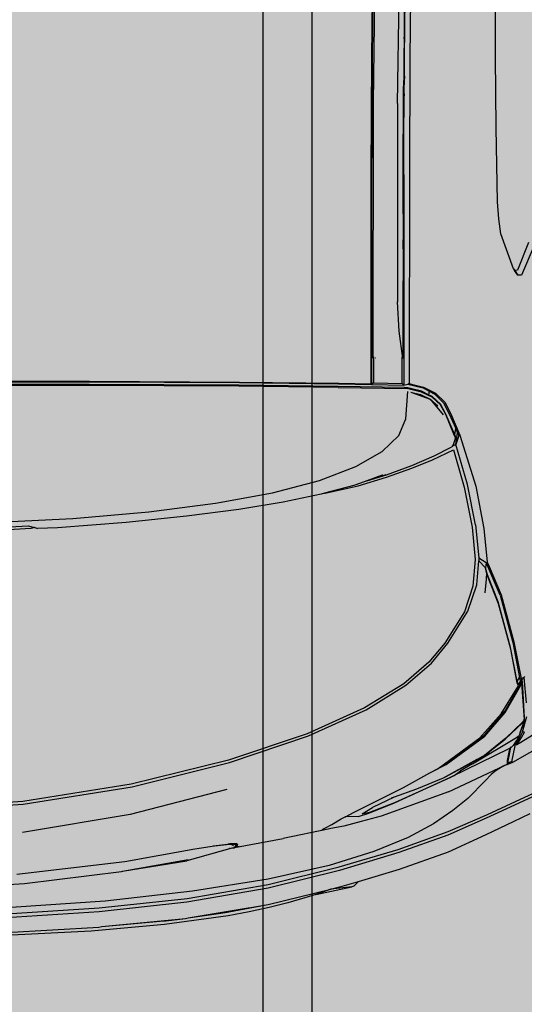
# Model space of a CAD drawing. Units: inches. Extents: x 1884 to 2398, y 474 to 1488.
# Tile 21 of 39: x 2330 to 2352, y 577 to 620. Entities that reach past the tile are written whole.
import ezdxf

# ---------------------------------------------------------------- set-up
doc = ezdxf.new("R2010")
doc.units = ezdxf.units.IN
doc.header["$MEASUREMENT"] = 0
doc.layers.get('0').update_dxf_attribs({"color": 250})
doc.layers.add('A-ANNO-DIMS', color=2, linetype='Continuous', lineweight=18)
doc.layers.add('C-VEHI', color=8, linetype='Continuous', lineweight=18)
doc.layers.add('Edges', color=250, linetype='Continuous')
doc.layers.add('L-PVMT-PATT', color=9, linetype='Continuous', lineweight=13, true_color=0xc7c8ca)
doc.styles.get("Standard").update_dxf_attribs({"font": 'arial.ttf'})
doc.dimstyles.get("Standard").update_dxf_attribs({"dimtxt": 7, "dimasz": 0.18, "dimexe": 0.18, "dimexo": 0.0625, "dimgap": 0.09, "dimtad": 0, "dimtih": 1, "dimtoh": 1, "dimzin": 0, "dimdsep": 46, "dimlunit": 3, "dimtxsty": 'Standard', "dimcen": 0.09, "dimadec": 0, "dimazin": 0, "dimtfac": 1, "dimtofl": 0, "dimtmove": 0, "dimatfit": 3, "dimfxl": 1, "dimtolj": 1, "dimtzin": 0, "dimarcsym": 0})

# ---------------------------------------------------------------- blocks, each defined once
blk = doc.blocks.new('Nissan Qashqai pl')
at = {"layer": 'Edges'}
for p, q in [((11.417, 12.6499), (11.4529, 12.5922)), ((11.4732, 12.585), (11.4462, 12.6324)), ((10.9059, 12.6087), (10.9384, 12.5945)), ((11.5165, 12.5882), (11.5074, 12.608)), ((11.5113, 12.6068), (11.5206, 12.5869)), ((10.9026, 12.6025), (10.933, 12.5901)), ((11.3792, 12.5982), (11.3804, 12.5972)), ((11.3804, 12.5972), (11.4082, 12.5998)), ((11.3827, 12.5953), (11.3804, 12.5972)), ((11.3811, 12.5958), (11.3808, 12.5961)), ((11.3834, 12.5947), (11.3827, 12.5953)), ((11.3846, 12.5953), (11.3829, 12.5952)), ((11.3829, 12.5952), (11.3849, 12.5951)), ((11.388, 12.591), (11.3829, 12.5952)), ((11.3846, 12.5953), (11.4248, 12.5976)), ((11.3846, 12.5953), (11.3846, 12.5953)), ((11.3851, 12.5951), (11.3846, 12.5953)), ((11.3846, 12.5953), (11.3849, 12.5951)), ((11.3849, 12.5951), (11.3851, 12.5951)), ((11.3882, 12.5923), (11.3849, 12.5951)), ((11.3851, 12.5951), (11.3867, 12.5949)), ((11.4171, 12.5766), (11.3851, 12.5951)), ((11.3867, 12.5949), (11.3915, 12.5951)), ((11.3915, 12.5951), (11.4266, 12.5977)), ((11.44, 12.5959), (11.423, 12.6006)), ((11.4248, 12.5976), (11.4266, 12.5977)), ((11.4266, 12.5977), (11.4252, 12.598)), ((11.4266, 12.5977), (11.4268, 12.5977)), ((11.4268, 12.5977), (11.4296, 12.5954)), ((11.4268, 12.5977), (11.4278, 12.5977)), ((11.4303, 12.5956), (11.4278, 12.5977)), ((11.4278, 12.5977), (11.43, 12.5969)), ((11.4296, 12.5954), (11.4469, 12.5773)), ((11.4337, 12.5962), (11.43, 12.5969)), ((11.43, 12.5969), (11.4361, 12.5948)), ((11.4479, 12.5766), (11.4303, 12.5956)), ((11.4397, 12.5937), (11.4337, 12.5962)), ((11.4403, 12.5978), (11.44, 12.5959)), ((11.44, 12.5959), (11.4457, 12.5928)), ((11.4462, 12.5947), (11.4403, 12.5978)), ((11.5384, 12.5859), (11.5295, 12.6041)), ((10.9316, 12.586), (10.8932, 12.572)), ((10.9316, 12.586), (10.9334, 12.5872)), ((10.932, 12.5862), (10.9316, 12.586)), ((10.9335, 12.5871), (10.932, 12.5862)), ((10.933, 12.5901), (10.9334, 12.5872)), ((10.9334, 12.5872), (10.9386, 12.5905)), ((10.9334, 12.5872), (10.9335, 12.5871)), ((10.9386, 12.5905), (10.9335, 12.5871)), ((10.9384, 12.5945), (10.9386, 12.5905)), ((11.2895, 12.5724), (11.3411, 12.5863)), ((11.29, 12.5711), (11.3419, 12.585)), ((11.3411, 12.5863), (11.3795, 12.5939)), ((11.3419, 12.585), (11.3804, 12.5926)), ((11.3847, 12.5899), (11.3474, 12.5827)), ((11.3863, 12.5898), (11.3493, 12.5828)), ((11.3795, 12.5939), (11.3834, 12.5947)), ((11.3804, 12.5926), (11.3841, 12.5933)), ((11.3847, 12.5899), (11.3804, 12.5926)), ((11.3834, 12.5947), (11.3841, 12.5933)), ((11.3847, 12.5899), (11.3848, 12.5899)), ((11.388, 12.591), (11.3848, 12.5899)), ((11.3895, 12.5912), (11.3863, 12.5898)), ((11.3914, 12.5926), (11.3867, 12.5949)), ((11.3886, 12.5919), (11.3872, 12.5927)), ((11.3882, 12.5923), (11.3886, 12.5919)), ((11.3886, 12.5919), (11.3895, 12.5912)), ((11.3892, 12.5916), (11.3886, 12.5919)), ((11.3923, 12.5894), (11.3895, 12.5912)), ((11.4187, 12.5768), (11.3914, 12.5926)), ((11.4203, 12.5724), (11.3923, 12.5894)), ((11.4361, 12.5948), (11.4406, 12.5932)), ((11.4406, 12.5932), (11.4397, 12.5937)), ((11.4406, 12.5932), (11.4442, 12.592)), ((11.4442, 12.592), (11.4497, 12.589)), ((11.4462, 12.5893), (11.4442, 12.592)), ((11.4457, 12.5928), (11.4512, 12.5893)), ((11.452, 12.591), (11.4462, 12.5947)), ((11.475, 12.5409), (11.4462, 12.5893)), ((11.4497, 12.589), (11.4498, 12.5889)), ((11.4535, 12.5876), (11.4498, 12.5889)), ((11.4498, 12.5889), (11.4549, 12.5855)), ((11.4512, 12.5893), (11.4535, 12.5876)), ((11.4539, 12.5897), (11.452, 12.591)), ((11.4529, 12.5922), (11.4542, 12.5894)), ((11.4535, 12.5876), (11.4532, 12.5882)), ((11.4535, 12.5876), (11.4542, 12.5894)), ((11.4535, 12.5876), (11.4728, 12.5838)), ((11.4542, 12.5894), (11.4539, 12.5897)), ((11.4549, 12.5855), (11.4568, 12.5836)), ((11.4732, 12.585), (11.4728, 12.5838)), ((11.4758, 12.5791), (11.4732, 12.585)), ((11.5306, 12.5573), (11.5165, 12.5882)), ((11.5206, 12.5869), (11.5349, 12.5559)), ((11.5527, 12.5559), (11.5384, 12.5859)), ((11.3474, 12.5827), (11.2972, 12.5692)), ((11.3493, 12.5828), (11.2993, 12.5695)), ((11.3474, 12.5827), (11.3474, 12.5827)), ((11.4433, 12.5543), (11.4171, 12.5766)), ((11.4447, 12.5545), (11.4187, 12.5768)), ((11.4469, 12.5773), (11.4659, 12.5539)), ((11.4654, 12.5548), (11.4479, 12.5766)), ((11.4564, 12.5833), (11.4567, 12.5833)), ((11.4569, 12.583), (11.4565, 12.5831)), ((11.4568, 12.5836), (11.4571, 12.5833)), ((11.4571, 12.5833), (11.4573, 12.583)), ((11.4573, 12.583), (11.4578, 12.5822)), ((11.4704, 12.5803), (11.4573, 12.583)), ((11.4573, 12.5823), (11.4574, 12.5822)), ((11.4573, 12.5823), (11.4573, 12.5823)), ((11.4576, 12.5822), (11.4574, 12.5822)), ((11.4578, 12.5822), (11.4588, 12.5807)), ((11.4605, 12.5816), (11.4578, 12.5822)), ((11.4588, 12.5807), (11.4895, 12.5178)), ((11.4713, 12.5794), (11.4605, 12.5816)), ((11.4742, 12.5797), (11.4704, 12.5803)), ((11.4744, 12.5792), (11.4713, 12.5794)), ((11.4728, 12.5838), (11.4742, 12.5797)), ((11.4728, 12.5838), (11.4746, 12.5796)), ((11.4742, 12.5797), (11.4744, 12.5792)), ((11.4745, 12.5797), (11.4742, 12.5797)), ((11.4745, 12.5792), (11.4744, 12.5792)), ((11.4745, 12.5792), (11.4745, 12.5797)), ((11.4745, 12.5797), (11.4746, 12.5796)), ((11.4748, 12.5792), (11.4745, 12.5792)), ((11.4746, 12.5796), (11.4748, 12.5792)), ((11.4746, 12.5796), (11.4758, 12.5791)), ((11.4758, 12.5791), (11.4748, 12.5792)), ((11.4758, 12.5791), (11.4759, 12.579)), ((11.4759, 12.579), (11.4778, 12.5746)), ((11.4759, 12.579), (11.4771, 12.576)), ((11.5057, 12.5145), (11.4771, 12.576)), ((11.4778, 12.5746), (11.4826, 12.5669)), ((10.6988, 12.5662), (10.5892, 12.5659)), ((10.7769, 12.5667), (10.6988, 12.5662)), ((10.858, 12.5683), (10.7769, 12.5667)), ((10.8766, 12.5697), (10.858, 12.5683)), ((10.8932, 12.572), (10.8766, 12.5697)), ((11.29, 12.5711), (11.2541, 12.5557)), ((11.2586, 12.5591), (11.2895, 12.5724)), ((11.2972, 12.5692), (11.2677, 12.5575)), ((11.2993, 12.5695), (11.2705, 12.5579)), ((11.4467, 12.5488), (11.4203, 12.5724)), ((11.4826, 12.5669), (11.4869, 12.5615)), ((11.1702, 12.5444), (11.2166, 12.5534)), ((11.2166, 12.5534), (11.2538, 12.5571)), ((11.2488, 12.548), (11.2541, 12.5557)), ((11.2599, 12.5552), (11.2524, 12.5477)), ((11.2538, 12.5571), (11.2586, 12.5591)), ((11.2541, 12.5557), (11.2599, 12.5552)), ((11.2677, 12.5575), (11.2599, 12.5552)), ((11.265, 12.5563), (11.2599, 12.5552)), ((11.2705, 12.5579), (11.265, 12.5563)), ((11.265, 12.5563), (11.2724, 12.5557)), ((11.2724, 12.5557), (11.2874, 12.5544)), ((11.4745, 12.5116), (11.4433, 12.5543)), ((11.4758, 12.5118), (11.4447, 12.5545)), ((11.4633, 12.5594), (11.4897, 12.5108)), ((11.4654, 12.5548), (11.4659, 12.5539)), ((11.4659, 12.5539), (11.4674, 12.5512)), ((11.4869, 12.5615), (11.4933, 12.555)), ((11.5131, 12.5356), (11.4933, 12.555)), ((11.5496, 12.5141), (11.5306, 12.5573)), ((11.5349, 12.5559), (11.5535, 12.5139)), ((11.5716, 12.5145), (11.5527, 12.5559)), ((11.1144, 12.5271), (11.1702, 12.5444)), ((11.2127, 12.5443), (11.1683, 12.5354)), ((11.2127, 12.5443), (11.2488, 12.548)), ((11.2152, 12.5404), (11.2509, 12.5439)), ((11.2488, 12.548), (11.2524, 12.5477)), ((11.2509, 12.5439), (11.28, 12.5414)), ((11.2785, 12.5455), (11.2524, 12.5477)), ((11.3076, 12.5358), (11.2785, 12.5455)), ((11.28, 12.5414), (11.3082, 12.532)), ((11.4801, 12.503), (11.4467, 12.5488)), ((11.4675, 12.551), (11.4674, 12.5512)), ((11.4675, 12.551), (11.4703, 12.546)), ((11.4703, 12.546), (11.4704, 12.5458)), ((11.4704, 12.5458), (11.4909, 12.5085)), ((11.4704, 12.5458), (11.4897, 12.5108)), ((11.475, 12.5409), (11.4828, 12.5276)), ((11.1683, 12.5354), (11.1244, 12.5227)), ((11.1302, 12.52), (11.1712, 12.5317)), ((11.1712, 12.5317), (11.2152, 12.5404)), ((11.3428, 12.5139), (11.3076, 12.5358)), ((11.3082, 12.532), (11.3425, 12.5106)), ((11.5131, 12.5356), (11.5265, 12.5194)), ((11.0902, 12.5166), (11.1144, 12.5271)), ((11.0908, 12.5153), (11.107, 12.5224)), ((11.1138, 12.5213), (11.0912, 12.5117)), ((11.1149, 12.5212), (11.0917, 12.5114)), ((11.107, 12.5224), (11.1116, 12.5243)), ((11.1138, 12.5213), (11.107, 12.5224)), ((11.1116, 12.5243), (11.1147, 12.5257)), ((11.1244, 12.5227), (11.1116, 12.5243)), ((11.1139, 12.5213), (11.1138, 12.5213)), ((11.1164, 12.5224), (11.1139, 12.5213)), ((11.1147, 12.5257), (11.1244, 12.5227)), ((11.1172, 12.5222), (11.1149, 12.5212)), ((11.1164, 12.5224), (11.1174, 12.5223)), ((11.1173, 12.5222), (11.1172, 12.5222)), ((11.1174, 12.5223), (11.1173, 12.5222)), ((11.12, 12.5215), (11.1174, 12.5223)), ((11.1246, 12.5199), (11.12, 12.5215)), ((11.1259, 12.5194), (11.1244, 12.5227)), ((11.1244, 12.5227), (11.126, 12.5194)), ((11.1259, 12.5194), (11.1246, 12.5199)), ((11.126, 12.5193), (11.1247, 12.5197)), ((11.126, 12.5193), (11.1248, 12.5195)), ((11.1251, 12.5189), (11.126, 12.5193)), ((11.126, 12.5193), (11.1259, 12.5194)), ((11.126, 12.5194), (11.1259, 12.5194)), ((11.126, 12.5194), (11.1261, 12.5193)), ((11.1264, 12.5192), (11.126, 12.5194)), ((11.1263, 12.5186), (11.126, 12.5193)), ((11.1261, 12.5193), (11.126, 12.5193)), ((11.1261, 12.5193), (11.1263, 12.5188)), ((11.1264, 12.5192), (11.1261, 12.5193)), ((11.1412, 12.4969), (11.1302, 12.52)), ((11.488, 12.5208), (11.4828, 12.5276)), ((11.5179, 12.4551), (11.488, 12.5208)), ((11.5265, 12.5194), (11.541, 12.4982)), ((11.0682, 12.5004), (11.0779, 12.5103)), ((11.0692, 12.4996), (11.0787, 12.5092)), ((11.0747, 12.4944), (11.092, 12.5087)), ((11.0779, 12.5103), (11.0902, 12.5166)), ((11.0787, 12.5092), (11.0908, 12.5153)), ((11.0912, 12.5117), (11.0802, 12.5057)), ((11.0917, 12.5114), (11.0809, 12.5056)), ((11.1277, 12.5167), (11.1264, 12.5192)), ((11.1369, 12.4986), (11.1277, 12.5167)), ((11.3425, 12.5106), (11.3635, 12.4929)), ((11.3645, 12.4958), (11.3428, 12.5139)), ((11.4788, 12.5052), (11.4745, 12.5116)), ((11.4852, 12.494), (11.4758, 12.5118)), ((11.4898, 12.5172), (11.4895, 12.5178)), ((11.4897, 12.5108), (11.4909, 12.5085)), ((11.4898, 12.5172), (11.49, 12.5167)), ((11.49, 12.5167), (11.5179, 12.4551)), ((11.4909, 12.5085), (11.5028, 12.4792)), ((11.5057, 12.5145), (11.5325, 12.4404)), ((11.5691, 12.4592), (11.5496, 12.5141)), ((11.5535, 12.5139), (11.5726, 12.46)), ((11.5908, 12.4606), (11.5716, 12.5145)), ((11.0614, 12.4872), (11.0682, 12.5004)), ((11.0658, 12.4932), (11.0692, 12.4996)), ((11.0802, 12.5057), (11.0718, 12.4967)), ((11.0809, 12.5056), (11.0727, 12.4966)), ((11.0747, 12.4944), (11.0821, 12.5029)), ((11.1475, 12.4741), (11.1369, 12.4986)), ((11.4801, 12.503), (11.4788, 12.5052)), ((11.4852, 12.494), (11.4801, 12.503)), ((11.541, 12.4982), (11.5562, 12.4701)), ((11.0581, 12.4738), (11.0614, 12.4872)), ((11.0624, 12.4866), (11.0658, 12.4932)), ((11.0658, 12.4932), (11.0698, 12.4925)), ((11.0698, 12.4925), (11.0659, 12.4848)), ((11.0727, 12.4966), (11.0669, 12.4849)), ((11.0671, 12.4731), (11.0747, 12.4944)), ((11.0696, 12.4836), (11.0747, 12.4944)), ((11.0718, 12.4967), (11.0698, 12.4925)), ((11.1505, 12.4742), (11.1412, 12.4969)), ((11.3635, 12.4929), (11.3872, 12.4654)), ((11.3888, 12.4678), (11.3645, 12.4958)), ((11.5013, 12.4651), (11.4852, 12.494)), ((11.0582, 12.47), (11.0624, 12.4866)), ((11.0659, 12.4848), (11.063, 12.4728)), ((11.0669, 12.4849), (11.0641, 12.4733)), ((11.0671, 12.4731), (11.0696, 12.4836)), ((11.5028, 12.4792), (11.5118, 12.4548)), ((10.7, 12.4662), (10.5566, 12.4677)), ((10.5572, 12.4737), (10.7004, 12.4722)), ((10.5576, 12.4675), (10.6649, 12.4659)), ((10.5866, 12.467), (10.6649, 12.4659)), ((10.6649, 12.4659), (10.6786, 12.4658)), ((10.6649, 12.4659), (10.6772, 12.4657)), ((10.6786, 12.4657), (10.6772, 12.4657)), ((10.6786, 12.4658), (10.6786, 12.4662)), ((10.6786, 12.4657), (10.6786, 12.4658)), ((10.6786, 12.4658), (10.6801, 12.4657)), ((10.6786, 12.4657), (10.6801, 12.4657)), ((10.6801, 12.4662), (10.6801, 12.4657)), ((10.6801, 12.4657), (10.6801, 12.4657)), ((10.6801, 12.4657), (10.6811, 12.4657)), ((10.6801, 12.4657), (10.6811, 12.4657)), ((10.6811, 12.4662), (10.6811, 12.4657)), ((10.6811, 12.4657), (10.6811, 12.4657)), ((10.6811, 12.4657), (10.6966, 12.4654)), ((10.6811, 12.4657), (10.6991, 12.4655)), ((10.6811, 12.4657), (10.6991, 12.4655)), ((10.6966, 12.4654), (10.7144, 12.4653)), ((10.6991, 12.4655), (10.7144, 12.4653)), ((10.7201, 12.4661), (10.7, 12.4662)), ((10.7004, 12.4722), (10.8279, 12.4715)), ((10.7144, 12.4653), (10.7239, 12.4653)), ((10.7201, 12.4661), (10.7306, 12.4653)), ((10.7395, 12.4659), (10.7201, 12.4661)), ((10.7239, 12.4653), (10.7248, 12.4653)), ((10.7306, 12.4653), (10.7248, 12.4653)), ((10.7311, 12.4652), (10.7306, 12.4653)), ((10.7495, 12.4652), (10.7311, 12.4652)), ((10.7311, 12.4652), (10.7502, 12.4651)), ((10.7395, 12.4659), (10.7495, 12.4652)), ((10.7923, 12.4656), (10.7395, 12.4659)), ((10.7923, 12.4652), (10.7923, 12.4656)), ((10.7933, 12.4656), (10.7923, 12.4656)), ((10.7933, 12.4652), (10.7933, 12.4656)), ((10.804, 12.4656), (10.7933, 12.4656)), ((10.804, 12.4653), (10.804, 12.4656)), ((10.8075, 12.4655), (10.804, 12.4656)), ((10.8075, 12.4655), (10.8075, 12.4653)), ((10.811, 12.4655), (10.8075, 12.4655)), ((10.811, 12.4655), (10.811, 12.4653)), ((10.8145, 12.4655), (10.811, 12.4655)), ((10.8145, 12.4653), (10.8145, 12.4655)), ((10.8279, 12.4654), (10.8145, 12.4655)), ((10.8279, 12.4715), (11.0544, 12.4714)), ((10.8279, 12.4654), (11.0592, 12.4653)), ((11.0544, 12.4714), (11.0575, 12.4714)), ((11.0574, 12.4637), (11.0592, 12.4653)), ((11.0575, 12.4714), (11.0581, 12.4738)), ((11.0575, 12.4714), (11.0582, 12.47)), ((11.0592, 12.4653), (11.0582, 12.47)), ((11.0585, 12.43), (11.0592, 12.4653)), ((11.0621, 12.4657), (11.0607, 12.3933)), ((11.0618, 12.3933), (11.0632, 12.47)), ((11.0622, 12.4697), (11.0621, 12.4657)), ((11.063, 12.4728), (11.0622, 12.4697)), ((11.0641, 12.4733), (11.0632, 12.47)), ((11.0962, 12.4675), (11.0662, 12.4698)), ((11.1148, 12.4598), (11.0962, 12.4675)), ((11.1577, 12.4465), (11.1475, 12.4741)), ((11.1605, 12.4465), (11.1505, 12.4742)), ((11.3872, 12.4654), (11.4138, 12.4223)), ((11.4159, 12.4242), (11.3888, 12.4678)), ((11.5562, 12.4701), (11.5715, 12.4326)), ((10.7502, 12.4586), (10.6237, 12.4603)), ((10.8179, 12.4648), (10.7495, 12.4652)), ((10.7502, 12.4651), (10.7504, 12.4651)), ((10.7502, 12.4586), (10.968, 12.4585)), ((10.7504, 12.4651), (10.7808, 12.4649)), ((10.7808, 12.4649), (10.8179, 12.4648)), ((10.8277, 12.4647), (10.8179, 12.4648)), ((10.8711, 12.4646), (10.8277, 12.4647)), ((10.8711, 12.4646), (10.8824, 12.4646)), ((10.8824, 12.4646), (10.8825, 12.4646)), ((10.8825, 12.4646), (10.8884, 12.4646)), ((10.8884, 12.4646), (10.8923, 12.4646)), ((10.8923, 12.4646), (10.8996, 12.4646)), ((10.9097, 12.4646), (10.8996, 12.4646)), ((10.9097, 12.4646), (10.9399, 12.4646)), ((10.9399, 12.4646), (10.9491, 12.4645)), ((10.9491, 12.4645), (11.0301, 12.4645)), ((11, 12.4605), (10.968, 12.4585)), ((11.0301, 12.4645), (11, 12.4605)), ((11.0301, 12.4637), (11.0287, 12.4637)), ((11.03, 12.4635), (11.0301, 12.4637)), ((11.0301, 12.4642), (11.0301, 12.4645)), ((11.0574, 12.4637), (11.0301, 12.4637)), ((11.0568, 12.4323), (11.0574, 12.4637)), ((11.1323, 12.4415), (11.1148, 12.4598)), ((11.5202, 12.427), (11.5013, 12.4651)), ((11.5118, 12.4548), (11.523, 12.4311)), ((11.5118, 12.4548), (11.513, 12.4514)), ((11.5292, 12.4272), (11.5179, 12.4551)), ((11.5179, 12.4551), (11.5285, 12.4279)), ((11.5884, 12.3943), (11.5691, 12.4592)), ((11.5726, 12.46), (11.5922, 12.3947)), ((11.6042, 12.4156), (11.5908, 12.4606)), ((11.1643, 12.425), (11.1576, 12.4459)), ((11.1643, 12.425), (11.1577, 12.4465)), ((11.1699, 12.4153), (11.1605, 12.4465)), ((10.6223, 12.4333), (10.7493, 12.4316)), ((11.0295, 12.4341), (11.0295, 12.4343)), ((11.1487, 12.4126), (11.1323, 12.4415)), ((11.1582, 12.4416), (11.1668, 12.4177)), ((11.1583, 12.4423), (11.1643, 12.425)), ((11.5325, 12.4404), (11.5386, 12.4187)), ((10.5561, 12.4323), (10.6996, 12.4308)), ((10.6999, 12.4304), (10.5563, 12.4318)), ((10.6996, 12.4308), (10.7722, 12.4304)), ((10.827, 12.4297), (10.6999, 12.4304)), ((10.7493, 12.4316), (11.0294, 12.4315)), ((10.7722, 12.4304), (10.7722, 12.4302)), ((10.7722, 12.4304), (10.7889, 12.4303)), ((10.7889, 12.4302), (10.7889, 12.4303)), ((10.7889, 12.4303), (10.7923, 12.4303)), ((10.7923, 12.4302), (10.7923, 12.4303)), ((10.7923, 12.4303), (10.7933, 12.4303)), ((10.7933, 12.4302), (10.7933, 12.4303)), ((10.7933, 12.4303), (10.8267, 12.4301)), ((10.8267, 12.4301), (11.0585, 12.43)), ((10.9133, 12.4296), (10.827, 12.4297)), ((10.9133, 12.4296), (10.9133, 12.4298)), ((10.9137, 12.4296), (10.9133, 12.4296)), ((10.9137, 12.4296), (10.9138, 12.4298)), ((10.9715, 12.4296), (10.9137, 12.4296)), ((10.9715, 12.4299), (10.9715, 12.4296)), ((11.0579, 12.4296), (10.9715, 12.4296)), ((11.0281, 12.4323), (11.0568, 12.4323)), ((11.0294, 12.4315), (11.0294, 12.4316)), ((11.0568, 12.4323), (11.0585, 12.43)), ((11.0572, 12.3942), (11.0579, 12.4296)), ((11.0579, 12.3938), (11.0585, 12.43)), ((11.0579, 12.4296), (11.0585, 12.43)), ((11.1643, 12.425), (11.1668, 12.4177)), ((11.4138, 12.4223), (11.4422, 12.3594)), ((11.4445, 12.3608), (11.4159, 12.4242)), ((11.5283, 12.4109), (11.5202, 12.427)), ((11.5301, 12.4198), (11.523, 12.4311)), ((11.5285, 12.4279), (11.5302, 12.4209)), ((11.5331, 12.4157), (11.5292, 12.4272)), ((11.5715, 12.4326), (11.5866, 12.3835)), ((11.164, 12.373), (11.1487, 12.4126)), ((11.1668, 12.4177), (11.1694, 12.4104)), ((11.178, 12.379), (11.1699, 12.4153)), ((11.5302, 12.4209), (11.5301, 12.4198)), ((11.5331, 12.4157), (11.5335, 12.401)), ((11.5386, 12.4187), (11.5434, 12.3997)), ((11.6042, 12.4156), (11.6077, 12.4125)), ((11.6103, 12.395), (11.6042, 12.4156)), ((11.6077, 12.4125), (11.6094, 12.4107)), ((11.1694, 12.4104), (11.1781, 12.3782)), ((11.5334, 12.4014), (11.5283, 12.4109)), ((11.5326, 12.4045), (11.5333, 12.4019)), ((11.5333, 12.4019), (11.5334, 12.4014)), ((11.5335, 12.401), (11.5334, 12.4014)), ((11.5357, 12.3968), (11.5335, 12.401)), ((11.6094, 12.4107), (11.6101, 12.4085)), ((11.6101, 12.4085), (11.6127, 12.3852)), ((11.6185, 12.3689), (11.6101, 12.4085)), ((11.056, 12.2851), (11.0572, 12.3942)), ((11.0566, 12.2849), (11.0579, 12.3938)), ((11.0607, 12.3933), (11.0595, 12.2842)), ((11.0618, 12.3933), (11.0606, 12.2841)), ((11.5416, 12.3863), (11.5357, 12.3968)), ((11.5434, 12.3997), (11.5461, 12.3854)), ((11.6076, 12.3166), (11.5884, 12.3943)), ((11.5922, 12.3947), (11.6118, 12.3165)), ((11.6127, 12.3852), (11.6103, 12.395)), ((11.1781, 12.3782), (11.178, 12.379)), ((11.5455, 12.3793), (11.5416, 12.3863)), ((11.5472, 12.3757), (11.5455, 12.3793)), ((11.5461, 12.3854), (11.5467, 12.3822)), ((11.5467, 12.3822), (11.5571, 12.3331)), ((11.5866, 12.3835), (11.6016, 12.3166)), ((11.6127, 12.3852), (11.6174, 12.3722)), ((11.6297, 12.3166), (11.6127, 12.3852)), ((11.1776, 12.3211), (11.164, 12.373)), ((11.1781, 12.3782), (11.1791, 12.3746)), ((11.1791, 12.3746), (11.1877, 12.333)), ((11.6174, 12.3722), (11.6185, 12.3689)), ((11.6185, 12.3689), (11.6224, 12.3567)), ((11.4422, 12.3594), (11.4712, 12.2729)), ((11.4738, 12.274), (11.4445, 12.3608)), ((11.6224, 12.3567), (11.6277, 12.3379)), ((11.6277, 12.3379), (11.6328, 12.3174)), ((11.1877, 12.333), (11.1958, 12.2844)), ((11.5668, 12.2816), (11.5571, 12.3331)), ((11.1891, 12.2586), (11.1776, 12.3211)), ((11.6016, 12.3166), (11.615, 12.2333)), ((11.6229, 12.2274), (11.6076, 12.3166)), ((11.6118, 12.3165), (11.6272, 12.2272)), ((11.6301, 12.3141), (11.6297, 12.3166)), ((11.6377, 12.2734), (11.6301, 12.3141)), ((11.6332, 12.2951), (11.6301, 12.3141)), ((11.6328, 12.3174), (11.6375, 12.2956)), ((11.6334, 12.2946), (11.6332, 12.2951)), ((11.6443, 12.2288), (11.6334, 12.2946)), ((11.6375, 12.2956), (11.6422, 12.2725)), ((11.0551, 12.1203), (11.056, 12.2851)), ((11.0557, 12.1202), (11.0566, 12.2849)), ((11.0595, 12.2842), (11.0586, 12.1198)), ((11.0606, 12.2841), (11.0597, 12.1196)), ((11.1958, 12.2844), (11.2033, 12.2269)), ((11.5626, 12.2771), (11.5627, 12.2817)), ((11.5627, 12.2817), (11.5634, 12.2829)), ((11.5627, 12.2817), (11.5633, 12.2814)), ((11.5632, 12.2783), (11.5633, 12.2814)), ((11.5633, 12.2814), (11.5634, 12.2829)), ((11.5633, 12.2814), (11.5661, 12.2803)), ((11.5634, 12.2829), (11.5668, 12.2816)), ((11.566, 12.2846), (11.5668, 12.2816)), ((11.5668, 12.2816), (11.5672, 12.2796)), ((11.4712, 12.2729), (11.4976, 12.1662)), ((11.5005, 12.167), (11.4738, 12.274)), ((11.5033, 12.271), (11.5307, 12.165)), ((11.5627, 12.2746), (11.5626, 12.2771)), ((11.5626, 12.2745), (11.5627, 12.2746)), ((11.5628, 12.2721), (11.5627, 12.2746)), ((11.5636, 12.2706), (11.5632, 12.2783)), ((11.5639, 12.2809), (11.5637, 12.2764)), ((11.5637, 12.2763), (11.5637, 12.2764)), ((11.5637, 12.2764), (11.5638, 12.2762)), ((11.5638, 12.2762), (11.5641, 12.2688)), ((11.5643, 12.2808), (11.5639, 12.2809)), ((11.5642, 12.2771), (11.5646, 12.2778)), ((11.566, 12.2801), (11.5643, 12.2808)), ((11.5647, 12.278), (11.5649, 12.2783)), ((11.566, 12.2801), (11.5661, 12.2803)), ((11.5662, 12.28), (11.566, 12.2801)), ((11.5661, 12.2803), (11.5662, 12.28)), ((11.5662, 12.28), (11.5661, 12.2803)), ((11.5669, 12.2797), (11.5661, 12.2803)), ((11.5669, 12.2797), (11.5662, 12.28)), ((11.5662, 12.28), (11.5662, 12.28)), ((11.5667, 12.2813), (11.567, 12.2796)), ((11.567, 12.2796), (11.5669, 12.2797)), ((11.5672, 12.2796), (11.567, 12.2796)), ((11.5678, 12.2766), (11.5672, 12.2796)), ((11.5673, 12.2784), (11.5677, 12.2767)), ((11.5678, 12.2766), (11.5818, 12.227)), ((11.5682, 12.2743), (11.5682, 12.2742)), ((11.5683, 12.2739), (11.5683, 12.2739)), ((11.5683, 12.2738), (11.5683, 12.2737)), ((11.6378, 12.2728), (11.6377, 12.2734)), ((11.6381, 12.2716), (11.6378, 12.2728)), ((11.639, 12.2645), (11.6378, 12.2728)), ((11.639, 12.2645), (11.6381, 12.2716)), ((11.6422, 12.2725), (11.6514, 12.2026)), ((11.565, 12.2577), (11.5636, 12.2706)), ((11.5641, 12.2688), (11.5656, 12.2559)), ((11.6443, 12.2288), (11.639, 12.2645)), ((11.1984, 12.1855), (11.1891, 12.2586)), ((11.5685, 12.2359), (11.565, 12.2577)), ((11.5823, 12.1589), (11.5685, 12.2359)), ((11.593, 12.1566), (11.58, 12.2288)), ((11.615, 12.2333), (11.626, 12.1375)), ((11.6333, 12.131), (11.6229, 12.2274)), ((11.6446, 12.2271), (11.6443, 12.2288)), ((11.2033, 12.2269), (11.21, 12.1607)), ((11.5883, 12.186), (11.5816, 12.2272)), ((11.5883, 12.186), (11.5818, 12.227)), ((11.6272, 12.2272), (11.6377, 12.1308)), ((11.6448, 12.2258), (11.6446, 12.2271)), ((11.6474, 12.2042), (11.6448, 12.2258)), ((11.6539, 12.1338), (11.6448, 12.2258)), ((11.6474, 12.2038), (11.6474, 12.2042)), ((11.6475, 12.2032), (11.6474, 12.2038)), ((11.648, 12.198), (11.6475, 12.2032)), ((11.6539, 12.1338), (11.648, 12.198)), ((11.6514, 12.2026), (11.6589, 12.1222)), ((11.2057, 12.1019), (11.1984, 12.1855)), ((11.593, 12.1566), (11.5883, 12.186)), ((11.4976, 12.1662), (11.5166, 12.0471)), ((11.5196, 12.0475), (11.5005, 12.167)), ((11.5307, 12.165), (11.5504, 12.0466)), ((11.21, 12.1607), (11.2159, 12.085)), ((11.5963, 12.0406), (11.5823, 12.1589)), ((11.5932, 12.1556), (11.593, 12.1566)), ((11.6067, 12.0489), (11.5932, 12.1556)), ((11.626, 12.1375), (11.6329, 12.0344)), ((11.6399, 12.029), (11.6333, 12.131)), ((11.6377, 12.1308), (11.6444, 12.0289)), ((11.6543, 12.1306), (11.6539, 12.1338)), ((11.6604, 12.0287), (11.6543, 12.1306)), ((11.0547, 11.9221), (11.0551, 12.1203)), ((11.0554, 11.9221), (11.0557, 12.1202)), ((11.0586, 12.1198), (11.0583, 11.9221)), ((11.0597, 12.1196), (11.0594, 11.9221)), ((11.6589, 12.1222), (11.6635, 12.0274)), ((11.2101, 12.012), (11.2057, 12.1019)), ((11.2159, 12.085), (11.2166, 12.063)), ((11.2139, 12.0528), (11.2158, 12.0599)), ((11.2158, 12.0602), (11.2166, 12.063)), ((11.2158, 12.0602), (11.2168, 12.056)), ((11.2158, 12.0599), (11.2158, 12.0602)), ((11.2158, 12.0599), (11.2168, 12.056)), ((11.2168, 12.056), (11.2204, 11.989)), ((11.2174, 11.9874), (11.2139, 12.0528)), ((11.5166, 12.0471), (11.5239, 11.9221)), ((11.527, 11.9221), (11.5196, 12.0475)), ((11.6133, 11.9221), (11.6067, 12.0489))]:
    blk.add_line(p, q, dxfattribs=at)
blk = doc.blocks.new('car')
blk.add_blockref('Nissan Qashqai pl', (-9.7433, -11.9151))
blk = doc.blocks.new('carr')
blk.add_blockref('car', (0.5124, -0.007))
blk = doc.blocks.new('*D23')
at = {"layer": 'A-ANNO-DIMS', "color": 0, "lineweight": -2, "transparency": 16777216}
for p, q in [((2272.304, 752.812), (2298.291, 752.812)), ((2298.111, 752.632), (2298.111, 670.29)), ((2298.111, 580.529), (2298.111, 662.871)), ((2272.304, 580.349), (2298.291, 580.349))]:
    blk.add_line(p, q, dxfattribs=at)
at = {"layer": 'A-ANNO-DIMS', "color": 0, "lineweight": 100, "transparency": 16777216}
for points in [[(2298.081, 752.632), (2298.141, 752.632), (2298.111, 752.812)], [(2298.081, 580.529), (2298.141, 580.529), (2298.111, 580.349)]]:
    blk.add_solid(points, dxfattribs=at)
at = {"layer": 'Defpoints', "color": 0, "lineweight": 100, "transparency": 16777216}
for p in [(2272.242, 752.812), (2272.242, 580.349), (2298.111, 580.349)]:
    blk.add_point(p, dxfattribs=at)
at = {"layer": 'A-ANNO-DIMS', "color": 0, "transparency": 16777216, "insert": (2298.111, 666.58), "char_height": 7, "attachment_point": 5}
blk.add_mtext('\\A1;CAR 14\'-4 1/2" TYP.', dxfattribs=at)
blk = doc.blocks.new('*D47')
at = {"layer": 'A-ANNO-DIMS', "color": 0, "lineweight": -2, "transparency": 16777216}
for p, q in [((2315.591, 959.704), (2315.591, 484.005)), ((2342.529, 959.704), (2342.529, 484.005)), ((2315.771, 484.185), (2319.606, 484.185)), ((2342.349, 484.185), (2338.513, 484.185))]:
    blk.add_line(p, q, dxfattribs=at)
at = {"layer": 'A-ANNO-DIMS', "color": 0, "lineweight": 100, "transparency": 16777216}
for points in [[(2315.771, 484.215), (2315.771, 484.155), (2315.591, 484.185)], [(2342.349, 484.215), (2342.349, 484.155), (2342.529, 484.185)]]:
    blk.add_solid(points, dxfattribs=at)
at = {"layer": 'Defpoints', "color": 0, "lineweight": 100, "transparency": 16777216}
for p in [(2315.591, 959.766), (2342.529, 959.766), (2342.529, 484.185)]:
    blk.add_point(p, dxfattribs=at)
at = {"layer": 'A-ANNO-DIMS', "color": 0, "transparency": 16777216, "insert": (2329.06, 484.185), "char_height": 7, "attachment_point": 5}
blk.add_mtext('\\A1;2\'-3"', dxfattribs=at)
blk = doc.blocks.new('*D49')
at = {"layer": 'A-ANNO-DIMS', "color": 0, "lineweight": -2, "transparency": 16777216}
for p, q in [((2318.409, 987.716), (2318.409, 484.005)), ((2340.409, 987.716), (2340.409, 484.005)), ((2318.589, 484.185), (2340.229, 484.185)), ((2340.409, 484.185), (2340.589, 484.185))]:
    blk.add_line(p, q, dxfattribs=at)
at = {"layer": 'A-ANNO-DIMS', "color": 0, "lineweight": 100, "transparency": 16777216}
for points in [[(2318.589, 484.215), (2318.589, 484.155), (2318.409, 484.185)], [(2340.229, 484.215), (2340.229, 484.155), (2340.409, 484.185)]]:
    blk.add_solid(points, dxfattribs=at)
at = {"layer": 'Defpoints', "color": 0, "lineweight": 100, "transparency": 16777216}
for p in [(2318.409, 987.778), (2340.409, 987.778), (2340.409, 484.185)]:
    blk.add_point(p, dxfattribs=at)
at = {"layer": 'A-ANNO-DIMS', "color": 0, "transparency": 16777216, "insert": (2352.373, 484.185), "char_height": 7, "attachment_point": 5}
blk.add_mtext('\\A1;1\'-10"', dxfattribs=at)

msp = doc.modelspace()

# ---------------------------------------------------------------- hatches: boundary and pattern name
at = {"layer": 'L-PVMT-PATT'}
h = msp.add_hatch(color=256, dxfattribs=at)
h.dxf.hatch_style = 1
h.paths.add_polyline_path([(2387.529, 769.966), (2351.529, 769.966), (2238.447, 769.966), (2238.447, 762.15), (2238.447, 754.445), (2126.529, 754.445), (2126.529, 676.183), (2134.868, 676.183), (2142.673, 676.183), (2142.673, 646.578), (2134.868, 646.578), (2126.529, 646.578), (2126.529, 640.17), (2387.529, 640.17)])
h.paths.add_polyline_path([(2387.529, 631.385), (2303.086, 631.385), (2303.086, 615.671), (2387.529, 615.671)])
h.paths.add_polyline_path([(2387.529, 640.17), (2126.529, 640.17), (2126.529, 631.385), (2387.529, 631.385)])
h.paths.add_polyline_path([(2393.529, 604.13), (2387.529, 604.13), (2387.529, 615.671), (2303.086, 615.671), (2303.086, 607.943), (2249.649, 607.943), (2126.529, 607.943), (2126.529, 533.885), (2393.529, 533.885)])
h.paths.add_polyline_path([(2257.825, 611.008), (2257.83, 611.337), (2257.915, 616.493), (2258.021, 621.805), (2258.146, 627.274), (2258.252, 631.385), (2126.529, 631.385), (2126.529, 611.008)])
h.paths.add_polyline_path([(2258.892, 611.285), (2258.888, 611.008), (2300.247, 611.008), (2300.247, 631.385), (2259.314, 631.385), (2259.206, 627.173), (2259.081, 621.72), (2258.976, 616.424)])

# ---------------------------------------------------------------- block references
at = {"layer": 'C-VEHI', "xscale": 39.37007874015748, "yscale": 39.37007874015748, "zscale": 39.37007874015748, "rotation": 270}
msp.add_blockref('carr', (2325.111, 676.232), dxfattribs=at)

# ---------------------------------------------------------------- dimensions: what is measured, and where the dimension line sits
at = {"layer": 'A-ANNO-DIMS'}
for base, p1, p2, picture, middle in [((2340.409, 484.185), (2318.409, 987.778), (2340.409, 987.778), '*D49', (2352.373, 484.185)), ((2342.529, 484.185), (2315.591, 959.766), (2342.529, 959.766), '*D47', (2329.06, 484.185))]:
    dim = msp.add_linear_dim(base=base, p1=p1, p2=p2, dimstyle='Standard', override={"dimdec": 1, "dimlfac": 1, "dimrnd": 0, "dimzin": 1, "dimdsep": 46, "dimlunit": 4, "dimfrac": 2}, dxfattribs=at)
    dim.commit()
    dim.dimension.update_dxf_attribs({"geometry": picture, "text_midpoint": middle})
dim = msp.add_linear_dim(base=(2298.111, 580.349), p1=(2272.242, 752.812), p2=(2272.242, 580.349), angle=270, text='CAR <> TYP.', dimstyle='Standard', override={"dimdec": 1, "dimlfac": 1, "dimrnd": 0, "dimzin": 1, "dimdsep": 46, "dimlunit": 4, "dimfrac": 2}, dxfattribs=at)
dim.commit()
dim.dimension.update_dxf_attribs({"geometry": '*D23', "text_midpoint": (2298.111, 666.58)})

doc.saveas('drawing.dxf')
